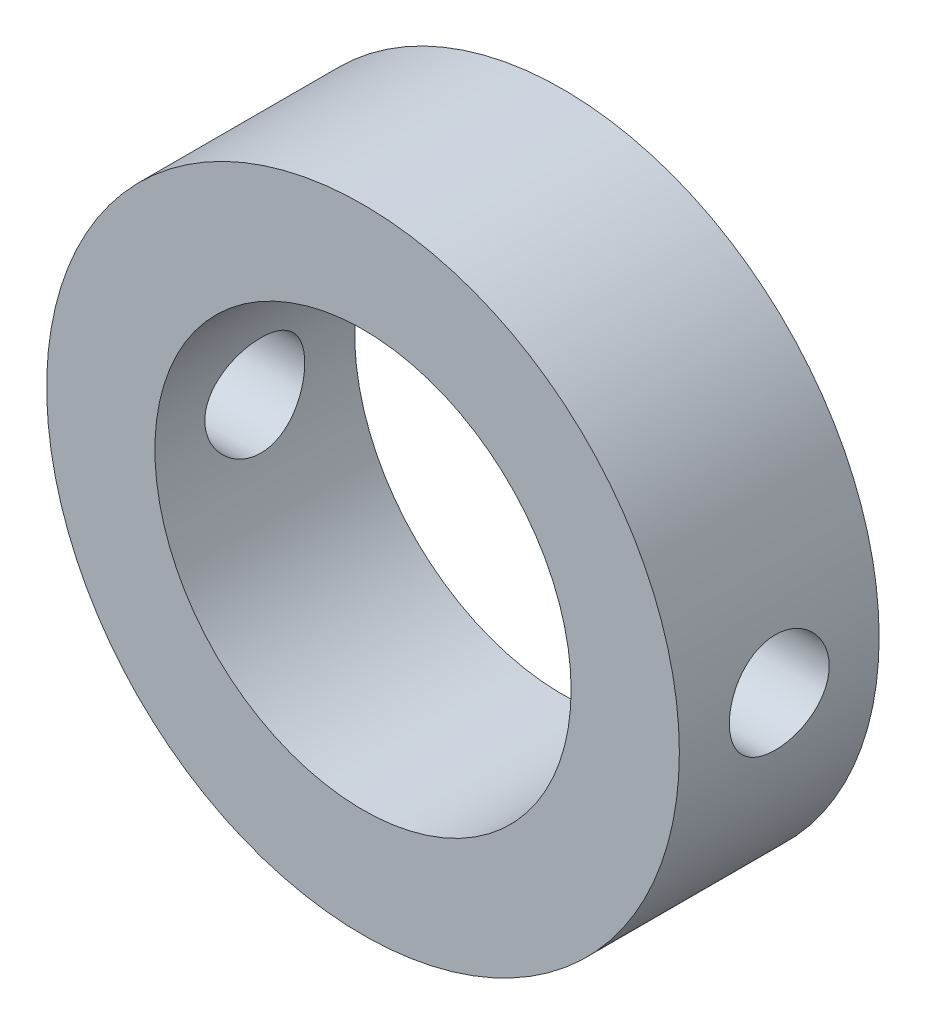
SolidWorks part; units mm, degrees
material "Plain Carbon Steel"
ref_plane "Front Plane" through (0, 0, 0) normal (0, 0, 1) x (1, 0, 0)
ref_plane "Top Plane" through (0, 0, 0) normal (0, 1, 0) x (1, 0, 0)
ref_plane "Right Plane" through (0, 0, 0) normal (1, 0, 0) x (0, 0, -1)
sketch "Collar Ring Profile" plane through (0, 0, 0) normal (0, 0, 1) x (1, 0, 0)
  circle A0 centre (0, 0) radius 12.5
  circle A1 centre (0, 0) radius 19
  dimension "D1" = 25
  dimension "D2" = 38
extrude "Collar Ring Ø38xØ25x12" add sketch "Collar Ring Profile" along normal blind 12
sketch "Cross Hole Profile" plane through (0, 0, 0) normal (1, 0, 0) x (0, 0, -1)
  line L0 (-12, 19) -> (-12, -19) construction
  circle A0 centre (-6, 0) radius 3
  dimension "D1" = 6
  dimension "D2" = 6
extrude "Cross Hole Ø6" cut sketch "Cross Hole Profile" against normal through all both and the other way through all contours A0
